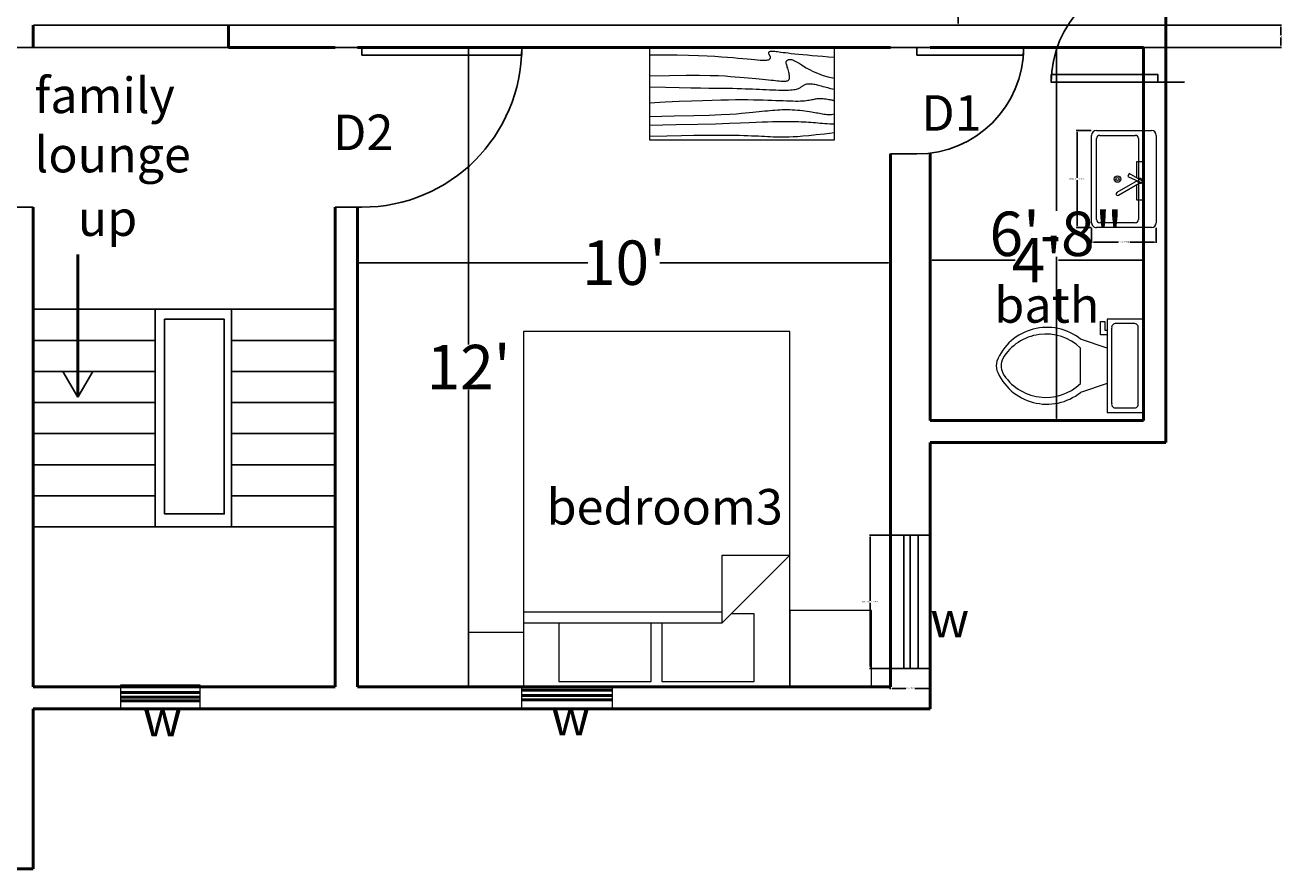
# Model space of a CAD drawing. Units: inches. Extents: x -10 to 557, y -66 to 886.
# Tile 5 of 6: x 210 to 493, y 497 to 687. Entities that reach past the tile are written whole.
import ezdxf

# ---------------------------------------------------------------- set-up
doc = ezdxf.new("R2010")
doc.units = ezdxf.units.IN
doc.header["$MEASUREMENT"] = 0
for name, color, linetype, lineweight in [('A-ANNO-DIMS', 2, 'Continuous', 18), ('A-ANNO-TEXT', 7, 'Continuous', 18), ('A-AREA-IDEN', 7, 'Continuous', 25), ('A-DOOR', 4, 'Continuous', 25), ('A-FLOR-FIXT', 8, 'Continuous', 18), ('A-FLOR-STRS', 3, 'Continuous', 25), ('A-FURN', 8, 'Continuous', 18), ('A-GLAZ', 4, 'Continuous', 25), ('A-WALL', 7, 'Continuous', 50)]:
    doc.layers.add(name, color=color, linetype=linetype, lineweight=lineweight)
doc.styles.get("Standard").update_dxf_attribs({"font": 'arial.ttf'})
doc.dimstyles.get("Standard").update_dxf_attribs({"dimtxt": 0.3, "dimasz": 0.4, "dimexe": 0.18, "dimexo": 0.0625, "dimgap": 0.09, "dimtad": 0, "dimtih": 1, "dimtoh": 1, "dimdec": 0, "dimrnd": 8, "dimzin": 0, "dimdsep": 46, "dimlunit": 3, "dimtxsty": 'Standard', "dimcen": 0.09, "dimadec": 0, "dimazin": 0, "dimtfac": 1, "dimtdec": 0, "dimtofl": 0, "dimtmove": 0, "dimatfit": 3, "dimfxl": 1, "dimtolj": 1, "dimtzin": 0, "dimarcsym": 0})

# ---------------------------------------------------------------- blocks, each defined once
blk = doc.blocks.new('*U4')
for p, q in [((0, 0), (0, -6)), ((24, 0), (24, -6))]:
    blk.add_line(p, q)
blk.add_lwpolyline([(0, 0), (0, 24), (1.75, 24), (1.75, 0)], close=True)
blk.add_arc((0, 0), 24, 0, 90)
blk = doc.blocks.new('*U5')
for p, q in [((0, 0), (0, -6)), ((-36, 0), (-36, -6))]:
    blk.add_line(p, q)
blk.add_lwpolyline([(0, 0), (0, 36), (-1.75, 36), (-1.75, 0)], close=True)
blk.add_arc((0, 0), 36, 90, 180)
blk = doc.blocks.new('Table - Rectangular Woodgrain 60 x 30 in.')
for p, q in [((0, 0), (0, -30)), ((60, 0), (0, 0)), ((60, -30), (60, 0)), ((0, -30), (60, -30))]:
    blk.add_line(p, q)
for points in [[(0, -2.4), (4.8155, -2.418), (9.0302, -2.4688), (12.709, -2.5477), (15.9167, -2.65), (18.7181, -2.7711), (21.1781, -2.9063), (23.3616, -3.0508), (25.3333, -3.2), (27.1477, -3.3495), (28.8172, -3.4958), (30.3437, -3.636), (31.7291, -3.7667), (32.9756, -3.8849), (34.0849, -3.9875), (35.059, -4.0714), (35.9, -4.1334), (36.6114, -4.1711), (37.2041, -4.1854), (37.6906, -4.1779), (38.0833, -4.15), (38.3948, -4.1034), (38.6375, -4.0396), (38.8239, -3.9602), (38.9666, -3.8667), (39.0764, -3.7608), (39.1573, -3.6448), (39.2116, -3.521), (39.2416, -3.3917), (39.2498, -3.2593), (39.2385, -3.1261), (39.21, -2.9944), (39.1666, -2.8667), (39.111, -2.7447), (39.0468, -2.6281), (38.978, -2.5163), (38.9083, -2.4083), (38.8418, -2.3035), (38.7823, -2.201), (38.7337, -2.1001), (38.7, -2), (38.6844, -1.9003), (38.6875, -1.8021), (38.7094, -1.707), (38.75, -1.6167), (38.8094, -1.5326), (38.8875, -1.4563), (38.9844, -1.3893), (39.1, -1.3333), (39.2351, -1.2896), (39.3937, -1.2583), (39.5804, -1.2396), (39.8, -1.2333), (40.057, -1.2396), (40.3562, -1.2583), (40.7023, -1.2896), (41.1, -1.3333), (41.5547, -1.3895), (42.0755, -1.4573), (42.6721, -1.5361), (43.3542, -1.625), (44.1316, -1.7233), (45.014, -1.8302), (46.0114, -1.9449), (47.1333, -2.0667), (48.3862, -2.1947), (49.7625, -2.3281), (51.2513, -2.4663), (52.8416, -2.6083), (54.5226, -2.7535), (56.2833, -2.9011), (58.1127, -3.0501), (60, -3.2)], [(0, -9.2), (6.5759, -9.0858), (11.9385, -9.0365), (16.2527, -9.0418), (19.6833, -9.0917), (22.3952, -9.1759), (24.5531, -9.2844), (26.322, -9.4069), (27.8666, -9.5333), (29.3241, -9.6553), (30.7203, -9.7719), (32.0532, -9.8837), (33.3208, -9.9917), (34.5213, -10.0965), (35.6526, -10.199), (36.7128, -10.2999), (37.7, -10.4), (38.6129, -10.4996), (39.4531, -10.5969), (40.223, -10.6895), (40.925, -10.775), (41.5613, -10.8512), (42.1344, -10.9156), (42.6465, -10.966), (43.1, -11), (43.4976, -11.0158), (43.8437, -11.0136), (44.143, -10.9942), (44.4, -10.9583), (44.6195, -10.9069), (44.8062, -10.8406), (44.9648, -10.7603), (45.1, -10.6667), (45.2155, -10.5598), (45.3114, -10.4365), (45.3871, -10.2929), (45.4416, -10.125), (45.4743, -9.929), (45.4844, -9.7011), (45.4709, -9.4371), (45.4333, -9.1333), (45.3716, -8.7883), (45.2896, -8.4104), (45.1919, -8.0107), (45.0833, -7.6), (44.9685, -7.1893), (44.8521, -6.7896), (44.7388, -6.4117), (44.6333, -6.0667), (44.54, -5.7628), (44.4614, -5.4979), (44.4001, -5.2675), (44.3583, -5.0667), (44.3384, -4.8909), (44.3427, -4.7354), (44.3736, -4.5956), (44.4333, -4.4667), (44.5236, -4.3453), (44.6427, -4.2333), (44.7884, -4.1339), (44.9583, -4.05), (45.1501, -3.9849), (45.3614, -3.9417), (45.59, -3.9234), (45.8333, -3.9333), (46.0915, -3.9749), (46.3734, -4.0531), (46.6906, -4.1736), (47.0542, -4.3417), (47.4756, -4.5629), (47.9661, -4.8427), (48.5372, -5.1866), (49.2, -5.6), (49.9676, -6.0844), (50.8594, -6.625), (51.8965, -7.2031), (53.1, -7.8), (54.491, -8.3969), (56.0906, -8.975), (57.9199, -9.5156), (60, -10)], [(0, -12.8), (5.1847, -12.9322), (9.6213, -13.0323), (13.3963, -13.1059), (16.5958, -13.1583), (19.3063, -13.1952), (21.614, -13.2219), (23.6054, -13.2439), (25.3666, -13.2667), (26.9728, -13.2947), (28.4531, -13.3281), (29.8256, -13.3663), (31.1083, -13.4083), (32.3191, -13.4535), (33.476, -13.501), (34.597, -13.5501), (35.7, -13.6), (36.7984, -13.6497), (37.8875, -13.6979), (38.9578, -13.743), (40, -13.7833), (41.0047, -13.8174), (41.9625, -13.8438), (42.864, -13.8607), (43.7, -13.8667), (44.4631, -13.8604), (45.1552, -13.8417), (45.7801, -13.8104), (46.3416, -13.7667), (46.8439, -13.7104), (47.2906, -13.6417), (47.6858, -13.5604), (48.0333, -13.4667), (48.3375, -13.3608), (48.6042, -13.2448), (48.8396, -13.121), (49.05, -12.9917), (49.2417, -12.8593), (49.4208, -12.7261), (49.5937, -12.5944), (49.7667, -12.4667), (49.9452, -12.3451), (50.1323, -12.2313), (50.3303, -12.1268), (50.5416, -12.0333), (50.7686, -11.9524), (51.0135, -11.8854), (51.2788, -11.8341), (51.5666, -11.8), (51.8785, -11.7843), (52.2116, -11.7865), (52.562, -11.8059), (52.926, -11.8417), (53.2998, -11.8931), (53.6795, -11.9594), (54.0614, -12.0397), (54.4416, -12.1333), (54.8223, -12.2401), (55.2293, -12.3625), (55.6942, -12.5037), (56.2489, -12.6667), (56.9251, -12.8547), (57.7545, -13.0708), (58.7689, -13.3182), (60, -13.6)], [(0, -18), (5.124, -17.7273), (9.6609, -17.5057), (13.6705, -17.3303), (17.2125, -17.1958), (20.3467, -17.0973), (23.1328, -17.0297), (25.6307, -16.9878), (27.9, -16.9667), (29.9928, -16.9617), (31.9302, -16.9703), (33.7254, -16.9907), (35.3917, -17.0208), (36.9423, -17.0588), (38.3906, -17.1026), (39.7499, -17.1503), (41.0333, -17.2), (42.2519, -17.2496), (43.4073, -17.2969), (44.4986, -17.3395), (45.525, -17.375), (46.4858, -17.4012), (47.3802, -17.4156), (48.2074, -17.416), (48.9667, -17.4), (49.6583, -17.3662), (50.2872, -17.3167), (50.8595, -17.2547), (51.3812, -17.1833), (51.8584, -17.1057), (52.2971, -17.025), (52.7034, -16.9443), (53.0833, -16.8667), (53.443, -16.7951), (53.789, -16.7313), (54.128, -16.6768), (54.4666, -16.6334), (54.8115, -16.6024), (55.1693, -16.5854), (55.5465, -16.5841), (55.95, -16.6), (56.3828, -16.6337), (56.8346, -16.6823), (57.2915, -16.7418), (57.7396, -16.8084), (58.165, -16.878), (58.5539, -16.9469), (58.8924, -17.0111), (59.1666, -17.0667), (59.3679, -17.1107), (59.5078, -17.1438), (59.6032, -17.1675), (59.6708, -17.1833), (59.7275, -17.193), (59.7901, -17.1979), (59.8753, -17.1998), (60, -17.2)], [(0, -22.4), (8.0098, -22.2501), (14.4094, -22.1011), (19.4168, -21.9535), (23.25, -21.8083), (26.1269, -21.6663), (28.2656, -21.5281), (29.884, -21.3947), (31.2, -21.2667), (32.3967, -21.1448), (33.5172, -21.0292), (34.5697, -20.9198), (35.5625, -20.8167), (36.5037, -20.7198), (37.4015, -20.6292), (38.2642, -20.5448), (39.1, -20.4667), (39.9164, -20.3951), (40.7187, -20.3313), (41.5117, -20.2768), (42.3, -20.2333), (43.0883, -20.2024), (43.8812, -20.1854), (44.6836, -20.1841), (45.5, -20.2), (46.3328, -20.234), (47.1747, -20.2844), (48.0163, -20.3488), (48.8479, -20.425), (49.66, -20.5106), (50.4429, -20.6031), (51.1872, -20.7004), (51.8833, -20.8), (52.5246, -20.8999), (53.1166, -20.9995), (53.6681, -21.0983), (54.1875, -21.1958), (54.6834, -21.2919), (55.1646, -21.3859), (55.6394, -21.4777), (56.1167, -21.5667), (56.6028, -21.6515), (57.0961, -21.7266), (57.5929, -21.7852), (58.0896, -21.8208), (58.5823, -21.8268), (59.0674, -21.7964), (59.5412, -21.723), (60, -21.6)], [(0, -25.2), (8.6355, -25.0504), (15.7026, -24.9031), (21.4049, -24.7606), (25.9458, -24.625), (29.529, -24.4988), (32.3578, -24.3844), (34.6359, -24.284), (36.5667, -24.2), (38.3213, -24.1341), (39.9417, -24.0854), (41.437, -24.0523), (42.8167, -24.0333), (44.0901, -24.0268), (45.2667, -24.0313), (46.3557, -24.0451), (47.3667, -24.0667), (48.309, -24.0947), (49.1928, -24.1287), (50.0284, -24.168), (50.826, -24.2125), (51.5959, -24.2617), (52.3483, -24.3151), (53.0935, -24.3725), (53.8417, -24.4334), (54.6009, -24.497), (55.3699, -24.561), (56.1454, -24.6226), (56.9239, -24.6792), (57.7021, -24.7279), (58.4764, -24.7662), (59.2435, -24.7911), (60, -24.8)], [(0, -28.8), (5.6867, -28.6681), (10.45, -28.5698), (14.407, -28.5012), (17.675, -28.4584), (20.3711, -28.4374), (22.6125, -28.4344), (24.5164, -28.4455), (26.2, -28.4667), (27.762, -28.4947), (29.2276, -28.5281), (30.6033, -28.5663), (31.8958, -28.6084), (33.1118, -28.6535), (34.2578, -28.7011), (35.3405, -28.7501), (36.3666, -28.8), (37.3443, -28.8497), (38.288, -28.8974), (39.2137, -28.9412), (40.1375, -28.9792), (41.0753, -29.0093), (42.0432, -29.0297), (43.0572, -29.0384), (44.1333, -29.0333), (45.2936, -29.0114), (46.5843, -28.9641), (48.0579, -28.8816), (49.7666, -28.7542), (51.7629, -28.5721), (54.0989, -28.3255), (56.8272, -28.0048), (60, -27.6)]]:
    blk.add_lwpolyline(points)
blk = doc.blocks.new('Bed - Queen')
for p, q in [((0, -80.00003), (0, 0)), ((0, 0), (59.99999, 0)), ((59.99999, 0), (59.99999, -80.00003)), ((7.99999, -1.2), (28.79998, -1.2)), ((7.99999, -14.4), (7.99999, -1.2)), ((28.79998, -1.2), (28.79998, -14.4)), ((31.19999, -1.2), (51.99999, -1.2)), ((31.19999, -14.4), (31.19999, -1.2)), ((51.99999, -1.2), (51.99999, -16.4)), ((0, -14.4), (44.8, -14.4)), ((44.8, -16.8), (0, -16.8)), ((59.99999, -29.6), (44.8, -14.4)), ((44.8, -14.4), (44.8, -29.6)), ((51.99999, -16.4), (46.79936, -16.4)), ((44.8, -29.6), (59.99999, -29.6)), ((59.99999, -80.00003), (0, -80.00003))]:
    blk.add_line(p, q)
blk = doc.blocks.new('Toilet - top')
for p, q in [((9.5, -6), (9.5, -2)), ((-8, -8.5), (-8, -8)), ((-7, -8), (-7, -9.5)), ((-4, -8), (-6, -14)), ((4, -8), (6, -14)), ((-10, -8.5), (-8, -8.5)), ((-10, -9.5), (-10, -8.5)), ((-7, -9.5), (-10, -9.5)), ((4, -14), (-4, -14))]:
    blk.add_line(p, q)
blk.add_lwpolyline([(10.5, -8), (10.5, 0), (-10.5, 0), (-10.5, -8)], close=True)
for points in [[(-9.5, -2), (-9.5, -6)], [(8.5, -1), (-8.5, -1)], [(-8.5, -7), (8.5, -7)]]:
    blk.add_lwpolyline(points)
for centre, radius, start, end in [((-8.62, -1.88), 0.884, 81.8699, 188.1301), ((8.62, -1.88), 0.884, 351.8699, 98.1301), ((-8.62, -6.12), 0.884, 171.8699, 278.1301), ((8.62, -6.12), 0.884, 261.8699, 8.1301), ((3.52, -21.58), 12.17, 141.4691, 247.9714), ((4.2, -21.82), 11.33, 136.3677, 238.9468), ((-3.52, -21.58), 12.17, 292.0284, 38.5307), ((-4.2, -21.82), 11.33, 301.053, 43.6321), ((0, -27.88), 4, 245.7318, 294.2682), ((0, -29), 4, 254.8605, 285.1395)]:
    blk.add_arc(centre, radius, start, end)
blk = doc.blocks.new('Sink-single - 30 in top')
blk.add_line((-15, -3.999996), (15, -3.999996))
for points in [[(-13.5, 0), (13.5, 0)], [(-15, -18.499996), (-15, -1.5)], [(15, -1.5), (15, -18.499996)], [(-13.5, -17.499996), (-13.5, -6.499996)], [(-12.5, -5.499996), (12.5, -5.499996)], [(13.5, -6.499996), (13.5, -17.499996)], [(12.5, -18.499996), (-12.5, -18.499996)], [(13.5, -19.999996), (-13.5, -19.999996)]]:
    blk.add_lwpolyline(points)
for radius in [1, 0.5]:
    blk.add_circle((0, -11.999996), radius)
for centre, radius, start, end in [((-13.5, -1.5), 1.5, 90, 180), ((13.5, -1.5), 1.5, 0, 90), ((-12.5, -6.499996), 1, 90, 180), ((12.5, -6.499996), 1, 0, 90), ((-13.5, -18.499996), 1.5, 180, 270), ((-12.5, -17.499996), 1, 180, 270), ((12.5, -17.499996), 1, 270, 0), ((13.5, -18.499996), 1.5, 270, 0)]:
    blk.add_arc(centre, radius, start, end)
blk = doc.blocks.new('Faucet - single handle top')
for p, q in [((0.08, -0.26), (-2.26, -4.34)), ((-1.37, -4.79), (0.55, -0.5)), ((-0.06, -1.9), (3.57, -8.18)), ((4.43, -7.68), (0.72, -1.24)), ((-2.26, -4.34), (-1.37, -4.79))]:
    blk.add_line(p, q)
for points in [[(-0.92, -2), (-6, -2), (-6, 0), (6, 0), (6, -2), (1.16, -2)], [(-0.01, -2), (-0.12, -2)]]:
    blk.add_lwpolyline(points)
for centre, radius, start, end in [((0, -1), 0.75, 269.2246, 216.2304), ((4, -7.93), 0.5, 210, 30)]:
    blk.add_arc(centre, radius, start, end)
blk = doc.blocks.new('*D22')
at = {"layer": 'A-ANNO-DIMS', "color": 0, "lineweight": -2, "transparency": 16777216}
for p, q in [((459.49, 802.16), (419.75, 802.16)), ((419.93, 801.76), (419.93, 747.31)), ((419.93, 687.56), (419.93, 742.02)), ((459.49, 687.16), (419.75, 687.16))]:
    blk.add_line(p, q, dxfattribs=at)
at = {"layer": 'A-ANNO-DIMS', "color": 0, "transparency": 16777216}
for points in [[(419.86, 801.76), (419.99, 801.76), (419.93, 802.16)], [(419.86, 687.56), (419.99, 687.56), (419.93, 687.16)]]:
    blk.add_solid(points, dxfattribs=at)
at = {"layer": 'Defpoints', "color": 0, "transparency": 16777216}
for p in [(459.55, 802.16), (419.93, 687.16), (459.55, 687.16)]:
    blk.add_point(p, dxfattribs=at)
at = {"layer": 'A-ANNO-DIMS', "color": 0, "transparency": 16777216, "insert": (419.93, 744.66), "char_height": 0.3, "attachment_point": 5}
blk.add_mtext('\\A1;{\\H16.66667x;9\'-4"}', dxfattribs=at)
blk = doc.blocks.new('*D23')
at = {"layer": 'A-ANNO-DIMS', "color": 0, "lineweight": -2, "transparency": 16777216}
for p, q in [((442.05, 681.8), (442.05, 645.39)), ((442.11, 682.2), (442.23, 682.2)), ((442.05, 598.6), (442.05, 635)), ((442.11, 598.2), (442.23, 598.2))]:
    blk.add_line(p, q, dxfattribs=at)
at = {"layer": 'A-ANNO-DIMS', "color": 0, "transparency": 16777216}
for points in [[(441.98, 681.8), (442.12, 681.8), (442.05, 682.2)], [(441.98, 598.6), (442.12, 598.6), (442.05, 598.2)]]:
    blk.add_solid(points, dxfattribs=at)
at = {"layer": 'Defpoints', "color": 0, "transparency": 16777216}
for p in [(442.05, 682.2), (442.05, 598.2), (442.05, 598.2)]:
    blk.add_point(p, dxfattribs=at)
at = {"layer": 'A-ANNO-DIMS', "color": 0, "transparency": 16777216, "insert": (442.05, 640.2), "char_height": 0.3, "attachment_point": 5}
blk.add_mtext('\\A1;{\\H33.33333x;6\'-8"}', dxfattribs=at)
blk = doc.blocks.new('*D24')
at = {"layer": 'A-ANNO-DIMS', "color": 0, "lineweight": -2, "transparency": 16777216}
for p, q in [((413.66, 632.08), (413.66, 634.43)), ((461.66, 632.08), (461.66, 634.43)), ((414.06, 634.25), (432.77, 634.25)), ((461.26, 634.25), (442.55, 634.25))]:
    blk.add_line(p, q, dxfattribs=at)
at = {"layer": 'A-ANNO-DIMS', "color": 0, "transparency": 16777216}
for points in [[(414.06, 634.32), (414.06, 634.18), (413.66, 634.25)], [(461.26, 634.32), (461.26, 634.18), (461.66, 634.25)]]:
    blk.add_solid(points, dxfattribs=at)
at = {"layer": 'Defpoints', "color": 0, "transparency": 16777216}
for p in [(413.66, 632.02), (461.66, 634.25), (461.66, 632.02)]:
    blk.add_point(p, dxfattribs=at)
at = {"layer": 'A-ANNO-DIMS', "color": 0, "transparency": 16777216, "insert": (437.66, 634.25), "char_height": 0.3, "attachment_point": 5}
blk.add_mtext("\\A1;{\\H33.33333x;4'}", dxfattribs=at)
blk = doc.blocks.new('*D25')
at = {"layer": 'A-ANNO-DIMS', "color": 0, "lineweight": -2, "transparency": 16777216}
for p, q in [((337.54, 682.2), (309.51, 682.2)), ((309.69, 681.8), (309.69, 615.31)), ((309.69, 538.6), (309.69, 605.09)), ((344.6, 538.2), (309.51, 538.2))]:
    blk.add_line(p, q, dxfattribs=at)
at = {"layer": 'A-ANNO-DIMS', "color": 0, "transparency": 16777216}
for points in [[(309.63, 681.8), (309.76, 681.8), (309.69, 682.2)], [(309.63, 538.6), (309.76, 538.6), (309.69, 538.2)]]:
    blk.add_solid(points, dxfattribs=at)
at = {"layer": 'Defpoints', "color": 0, "transparency": 16777216}
for p in [(337.61, 682.2), (309.69, 538.2), (344.66, 538.2)]:
    blk.add_point(p, dxfattribs=at)
at = {"layer": 'A-ANNO-DIMS', "color": 0, "transparency": 16777216, "insert": (309.69, 610.2), "char_height": 0.3, "attachment_point": 5}
blk.add_mtext("\\A1;{\\H33.33333x;12'}", dxfattribs=at)
blk = doc.blocks.new('*D26')
at = {"layer": 'A-ANNO-DIMS', "color": 0, "lineweight": -2, "transparency": 16777216}
for p, q in [((284.66, 636.24), (284.66, 633.52)), ((404.66, 636.24), (404.66, 633.52)), ((285.06, 633.7), (336.56, 633.7)), ((404.26, 633.7), (352.77, 633.7))]:
    blk.add_line(p, q, dxfattribs=at)
at = {"layer": 'A-ANNO-DIMS', "color": 0, "transparency": 16777216}
for points in [[(285.06, 633.76), (285.06, 633.63), (284.66, 633.7)], [(404.26, 633.76), (404.26, 633.63), (404.66, 633.7)]]:
    blk.add_solid(points, dxfattribs=at)
at = {"layer": 'Defpoints', "color": 0, "transparency": 16777216}
for p in [(284.66, 636.31), (404.66, 636.31), (404.66, 633.7)]:
    blk.add_point(p, dxfattribs=at)
at = {"layer": 'A-ANNO-DIMS', "color": 0, "transparency": 16777216, "insert": (344.66, 633.7), "char_height": 0.3, "attachment_point": 5}
blk.add_mtext("\\A1;{\\H33.33333x;10'}", dxfattribs=at)
blk = doc.blocks.new('*U31')
for p, q in [((0, 0), (0, -6)), ((24, 0), (24, -6))]:
    blk.add_line(p, q)
blk.add_lwpolyline([(0, 0), (0, 24), (1.75, 24), (1.75, 0)], close=True)
blk.add_arc((0, 0), 24, 0, 90)
blk = doc.blocks.new('WIN-900')
for p, q in [((0, 6.25), (30, 6.25)), ((0, 4.5), (30, 4.5)), ((0, 3.05), (30, 3.05))]:
    blk.add_line(p, q)
blk.add_lwpolyline([(0, 9), (0, 0), (30, 0), (30, 9)], close=True)
blk = doc.blocks.new('*D57')
at = {"layer": 'A-ANNO-DIMS', "color": 0, "lineweight": -2, "ltscale": 2, "transparency": 16777216}
for p, q in [((404.59, 572.33), (399.97, 572.33)), ((400.15, 571.93), (400.15, 557.57)), ((400.15, 542.73), (400.15, 557.08)), ((404.59, 542.33), (399.97, 542.33))]:
    blk.add_line(p, q, dxfattribs=at)
at = {"layer": 'A-ANNO-DIMS', "color": 0, "ltscale": 2, "transparency": 16777216}
for points in [[(400.08, 571.93), (400.22, 571.93), (400.15, 572.33)], [(400.08, 542.73), (400.22, 542.73), (400.15, 542.33)]]:
    blk.add_solid(points, dxfattribs=at)
at = {"layer": 'Defpoints', "color": 0, "ltscale": 2, "transparency": 16777216}
for p in [(404.65, 572.33), (400.15, 542.33), (404.65, 542.33)]:
    blk.add_point(p, dxfattribs=at)
at = {"layer": 'A-ANNO-DIMS', "color": 0, "ltscale": 2, "transparency": 16777216, "insert": (400.15, 557.33), "char_height": 0.3, "attachment_point": 5}
blk.add_mtext('\\A1;WINDOW 2\'-6" TYP.', dxfattribs=at)
blk = doc.blocks.new('*D58')
at = {"layer": 'A-ANNO-DIMS', "color": 0, "lineweight": -2, "ltscale": 2, "transparency": 16777216}
for p, q in [((404.65, 542.26), (404.65, 537.65)), ((413.65, 542.26), (413.65, 537.65)), ((405.05, 537.83), (408.15, 537.83)), ((413.25, 537.83), (410.16, 537.83))]:
    blk.add_line(p, q, dxfattribs=at)
at = {"layer": 'A-ANNO-DIMS', "color": 0, "ltscale": 2, "transparency": 16777216}
for points in [[(405.05, 537.89), (405.05, 537.76), (404.65, 537.83)], [(413.25, 537.89), (413.25, 537.76), (413.65, 537.83)]]:
    blk.add_solid(points, dxfattribs=at)
at = {"layer": 'Defpoints', "color": 0, "ltscale": 2, "transparency": 16777216}
for p in [(404.65, 542.33), (413.65, 542.33), (413.65, 537.83)]:
    blk.add_point(p, dxfattribs=at)
at = {"layer": 'A-ANNO-DIMS', "color": 0, "ltscale": 2, "transparency": 16777216, "insert": (409.15, 537.83), "char_height": 0.3, "attachment_point": 5}
blk.add_mtext('\\A1;0\'-9" TYP.', dxfattribs=at)
blk = doc.blocks.new('*D69')
at = {"layer": 'A-ANNO-DIMS', "color": 0, "lineweight": -2, "ltscale": 2, "transparency": 16777216}
for p, q in [((449.91, 663.48), (446.51, 663.48)), ((446.69, 663.08), (446.69, 652.79)), ((446.69, 642.01), (446.69, 652.3)), ((449.91, 641.61), (446.51, 641.61))]:
    blk.add_line(p, q, dxfattribs=at)
at = {"layer": 'A-ANNO-DIMS', "color": 0, "ltscale": 2, "transparency": 16777216}
for points in [[(446.63, 663.08), (446.76, 663.08), (446.69, 663.48)], [(446.63, 642.01), (446.76, 642.01), (446.69, 641.61)]]:
    blk.add_solid(points, dxfattribs=at)
at = {"layer": 'Defpoints', "color": 0, "ltscale": 2, "transparency": 16777216}
for p in [(449.97, 663.48), (446.69, 641.61), (449.97, 641.61)]:
    blk.add_point(p, dxfattribs=at)
at = {"layer": 'A-ANNO-DIMS', "color": 0, "ltscale": 2, "transparency": 16777216, "insert": (446.69, 652.54), "char_height": 0.3, "attachment_point": 5}
blk.add_mtext('\\A1;BASIN 1\'-10" TYP.', dxfattribs=at)
blk = doc.blocks.new('*D70')
at = {"layer": 'A-ANNO-DIMS', "color": 0, "lineweight": -2, "ltscale": 2, "transparency": 16777216}
for p, q in [((449.97, 641.55), (449.97, 638.15)), ((464.55, 641.55), (464.55, 638.15)), ((450.37, 638.33), (455.92, 638.33)), ((464.15, 638.33), (458.6, 638.33))]:
    blk.add_line(p, q, dxfattribs=at)
at = {"layer": 'A-ANNO-DIMS', "color": 0, "ltscale": 2, "transparency": 16777216}
for points in [[(450.37, 638.4), (450.37, 638.26), (449.97, 638.33)], [(464.15, 638.4), (464.15, 638.26), (464.55, 638.33)]]:
    blk.add_solid(points, dxfattribs=at)
at = {"layer": 'Defpoints', "color": 0, "ltscale": 2, "transparency": 16777216}
for p in [(449.97, 641.61), (464.55, 641.61), (464.55, 638.33)]:
    blk.add_point(p, dxfattribs=at)
at = {"layer": 'A-ANNO-DIMS', "color": 0, "ltscale": 2, "transparency": 16777216, "insert": (457.26, 638.33), "char_height": 0.3, "attachment_point": 5}
blk.add_mtext('\\A1;1\'-2 1/2" TYP.', dxfattribs=at)
blk = doc.blocks.new('*D80')
at = {"layer": 'A-ANNO-DIMS', "color": 0, "lineweight": -2, "ltscale": 2, "transparency": 16777216}
for p, q in [((211.73, 687.2), (492.77, 687.2)), ((492.59, 686.8), (492.59, 684.94)), ((492.59, 682.6), (492.59, 684.45)), ((211.73, 682.2), (492.77, 682.2))]:
    blk.add_line(p, q, dxfattribs=at)
at = {"layer": 'A-ANNO-DIMS', "color": 0, "ltscale": 2, "transparency": 16777216}
for points in [[(492.52, 686.8), (492.65, 686.8), (492.59, 687.2)], [(492.52, 682.6), (492.65, 682.6), (492.59, 682.2)]]:
    blk.add_solid(points, dxfattribs=at)
at = {"layer": 'Defpoints', "color": 0, "ltscale": 2, "transparency": 16777216}
for p in [(211.66, 687.2), (492.59, 687.2), (211.66, 682.2)]:
    blk.add_point(p, dxfattribs=at)
at = {"layer": 'A-ANNO-DIMS', "color": 0, "ltscale": 2, "transparency": 16777216, "insert": (492.59, 684.7), "char_height": 0.3, "attachment_point": 5}
blk.add_mtext('\\A1;0\'-5"', dxfattribs=at)

msp = doc.modelspace()

# ---------------------------------------------------------------- linework, layer by layer
at = {"layer": 'A-FLOR-STRS'}
for p, q in [((211.66, 623.2), (279.66, 623.2)), ((211.66, 616.2), (239.13, 616.2)), ((256.31, 616.2), (279.66, 616.2)), ((211.66, 609.2), (239.13, 609.2)), ((256.31, 609.2), (279.66, 609.2)), ((211.66, 602.2), (239.13, 602.2)), ((256.31, 602.2), (279.66, 602.2)), ((211.66, 595.2), (239.13, 595.2)), ((256.31, 595.2), (279.66, 595.2)), ((211.66, 588.2), (239.13, 588.2)), ((256.31, 588.2), (279.66, 588.2)), ((211.66, 581.2), (239.13, 581.2)), ((256.31, 581.2), (279.66, 581.2)), ((211.66, 574.2), (279.66, 574.2))]:
    msp.add_line(p, q, dxfattribs=at)
for points in [[(239.13, 623.2), (256.31, 623.2), (256.31, 574.2), (239.13, 574.2)], [(241.22, 620.98), (254.67, 620.98), (254.67, 577.14), (241.22, 577.14)], [(221.7, 603.39), (225.05, 609.2), (218.34, 609.2)]]:
    msp.add_lwpolyline(points, close=True, dxfattribs=at)
at = {"layer": 'A-FURN'}
for points in [[(382.02, 538.2), (400.39, 538.2), (400.39, 555.39), (382.02, 555.39)], [(322.02, 538.2), (309.69, 538.2), (309.69, 550.5), (322.02, 550.5)], [(231.28, 538.58), (231.28, 533.2), (249.24, 533.2), (249.24, 538.58)]]:
    msp.add_lwpolyline(points, close=True, dxfattribs=at)
msp.add_lwpolyline([(321.64, 538.2), (321.64, 533.2), (342.07, 533.2), (342.07, 538.2)], dxfattribs=at)
at = {"layer": 'A-WALL'}
for p, q in [((466.66, 682.2), (466.66, 807.2)), ((211.66, 682.2), (211.66, 687.2)), ((255.66, 687.2), (255.66, 682.2)), ((255.66, 682.2), (279.66, 682.2)), ((284.66, 682.2), (404.66, 682.2)), ((413.66, 682.2), (461.66, 682.2)), ((413.66, 682.2), (461.66, 682.2)), ((461.66, 682.2), (461.66, 598.2)), ((466.66, 682.2), (466.66, 593.2)), ((404.66, 658.2), (404.66, 538.2)), ((413.66, 658.38), (413.66, 598.2)), ((211.66, 538.2), (211.66, 646.2)), ((279.66, 646.2), (279.66, 538.2)), ((284.66, 646.2), (284.66, 538.2)), ((221.7, 635.52), (221.7, 603.52)), ((461.66, 598.2), (413.66, 598.2)), ((466.66, 593.2), (413.66, 593.2)), ((413.66, 593.2), (413.66, 533.2)), ((211.66, 538.2), (279.66, 538.2)), ((284.66, 538.2), (404.66, 538.2)), ((231.28, 536.94), (249.24, 536.94)), ((231.28, 535.89), (249.24, 535.89)), ((321.64, 537.46), (342.07, 537.46)), ((321.64, 536.26), (342.07, 536.26)), ((321.64, 535.27), (342.07, 535.27)), ((211.66, 497.2), (211.66, 533.2)), ((211.66, 533.2), (413.66, 533.2)), ((231.28, 535.02), (249.24, 535.02)), ((53.66, 497.2), (211.66, 497.2))]:
    msp.add_line(p, q, dxfattribs=at)

# ---------------------------------------------------------------- block references
at = {"layer": 'A-DOOR'}
for name, p, rotation in [('*U31', (464.89, 674.32), 90), ('*U5', (205.66, 682.2), 90), ('*U4', (410.66, 682.2), 270)]:
    msp.add_blockref(name, p, dxfattribs=dict(at, rotation=rotation))
at = {"layer": 'A-DOOR', "xscale": -1, "rotation": 270}
msp.add_blockref('*U5', (285.66, 682.2), dxfattribs=at)
at = {"layer": 'A-FLOR-FIXT', "xscale": 0.7289455405337706, "yscale": 0.7289455405337706, "zscale": 0.7289455405337706, "rotation": 270}
for name, p in [('Sink-single - 30 in top', (464.55, 652.54)), ('Faucet - single handle top', (461.62, 652.12))]:
    msp.add_blockref(name, p, dxfattribs=at)
at = {"layer": 'A-FLOR-FIXT', "rotation": 270}
msp.add_blockref('Toilet - top', (461.49, 610.49), dxfattribs=at)
at = {"layer": 'A-FURN', "xscale": 0.6942880543039835, "yscale": 0.6942880543039835, "zscale": 0.6942880543039835}
msp.add_blockref('Table - Rectangular Woodgrain 60 x 30 in.', (350.4, 682.2), dxfattribs=at)
msp.add_blockref('Table - Rectangular Woodgrain 60 x 30 in.', (350.4, 682.2), dxfattribs=at)
msp.add_blockref('Table - Rectangular Woodgrain 60 x 30 in.', (350.4, 682.2), dxfattribs=at)
msp.add_blockref('Table - Rectangular Woodgrain 60 x 30 in.', (350.4, 682.2), dxfattribs=at)
at = {"layer": 'A-FURN', "xscale": -1, "rotation": 180}
msp.add_blockref('Bed - Queen', (322.02, 538.2), dxfattribs=at)
at = {"layer": 'A-GLAZ', "rotation": 270.0000000000001}
msp.add_blockref('WIN-900', (404.65, 572.33), dxfattribs=at)

# ---------------------------------------------------------------- texts
at = {"layer": 'A-ANNO-TEXT', "char_height": 8, "attachment_point": 1}
for s, width, insert in [('D1', 13.506, (411.63, 671.42)), ('D2', 13.506, (279.18, 667.05)), ('up', 33.8308, (221.7, 647.73)), ('w', 13.506, (413.65, 557.33)), ('w', 13.506, (236.37, 535.02)), ('w', 13.506, (328.29, 535.27))]:
    msp.add_mtext_dynamic_manual_height_columns(s, width=width, gutter_width=1, heights=[0], dxfattribs=dict(at, insert=insert))
at = {"layer": 'A-AREA-IDEN', "char_height": 8, "attachment_point": 1}
for s, width, insert in [('family lounge', 67.0443, (211.96, 675.38)), ('bath', 38.1538, (428.08, 628.18)), ('bedroom3', 38.1538, (327.26, 582.74))]:
    msp.add_mtext_dynamic_manual_height_columns(s, width=width, gutter_width=1, heights=[0], dxfattribs=dict(at, insert=insert))

# ---------------------------------------------------------------- dimensions: what is measured, and where the dimension line sits
at = {"layer": 'A-ANNO-DIMS'}
for base, p1, p2, text, picture, middle in [((419.93, 687.16), (459.55, 802.16), (459.55, 687.16), '{\\H16.66667x;<>}', '*D22', (419.93, 744.66)), ((309.69, 538.2), (337.61, 682.2), (344.66, 538.2), '{\\H33.33333x;<>}', '*D25', (309.69, 610.2)), ((442.05, 598.2), (442.05, 682.2), (442.05, 598.2), '{\\H33.33333x;<>}', '*D23', (442.05, 640.2))]:
    dim = msp.add_linear_dim(base=base, p1=p1, p2=p2, angle=90, text=text, dimstyle='Standard', override={"dimclrd": 0, "dimclre": 0, "dimclrt": 0}, dxfattribs=at)
    dim.commit()
    dim.dimension.update_dxf_attribs({"geometry": picture, "text_midpoint": middle})
at = {"layer": 'A-ANNO-DIMS', "ltscale": 2}
dim = msp.add_linear_dim(base=(492.59, 687.2), p1=(211.66, 682.2), p2=(211.66, 687.2), angle=90, dimstyle='Standard', override={"dimdec": 1, "dimlfac": 1, "dimrnd": 0, "dimzin": 1, "dimdsep": 46, "dimlunit": 4, "dimfrac": 2}, dxfattribs=at)
dim.commit()
dim.dimension.update_dxf_attribs({"geometry": '*D80', "text_midpoint": (492.59, 684.7)})
for base, p1, p2, angle, text, picture, middle in [((446.69, 641.61), (449.97, 663.48), (449.97, 641.61), 270, 'BASIN <> TYP.', '*D69', (446.69, 652.54)), ((400.15, 542.33), (404.65, 572.33), (404.65, 542.33), 270, 'WINDOW <> TYP.', '*D57', (400.15, 557.33)), ((413.65, 537.83), (404.65, 542.33), (413.65, 542.33), 0, '<> TYP.', '*D58', (409.15, 537.83))]:
    dim = msp.add_linear_dim(base=base, p1=p1, p2=p2, angle=angle, text=text, dimstyle='Standard', override={"dimdec": 1, "dimrnd": 0, "dimzin": 1, "dimlunit": 4, "dimfrac": 2}, dxfattribs=at)
    dim.commit()
    dim.dimension.update_dxf_attribs({"geometry": picture, "text_midpoint": middle})
dim = msp.add_linear_dim(base=(464.55, 638.33), p1=(449.97, 641.61), p2=(464.55, 641.61), text='<> TYP.', dimstyle='Standard', override={"dimdec": 1, "dimrnd": 0, "dimzin": 1, "dimlunit": 4, "dimfrac": 2}, dxfattribs=at)
dim.commit()
dim.dimension.update_dxf_attribs({"geometry": '*D70', "text_midpoint": (457.26, 638.33)})
at = {"layer": 'A-ANNO-DIMS'}
for base, p1, p2, picture, middle in [((404.66, 633.7), (284.66, 636.31), (404.66, 636.31), '*D26', (344.66, 633.7)), ((461.66, 634.25), (413.66, 632.02), (461.66, 632.02), '*D24', (437.66, 634.25))]:
    dim = msp.add_linear_dim(base=base, p1=p1, p2=p2, text='{\\H33.33333x;<>}', dimstyle='Standard', override={"dimclrd": 0, "dimclre": 0, "dimclrt": 0}, dxfattribs=at)
    dim.commit()
    dim.dimension.update_dxf_attribs({"geometry": picture, "text_midpoint": middle})

doc.saveas('drawing.dxf')
